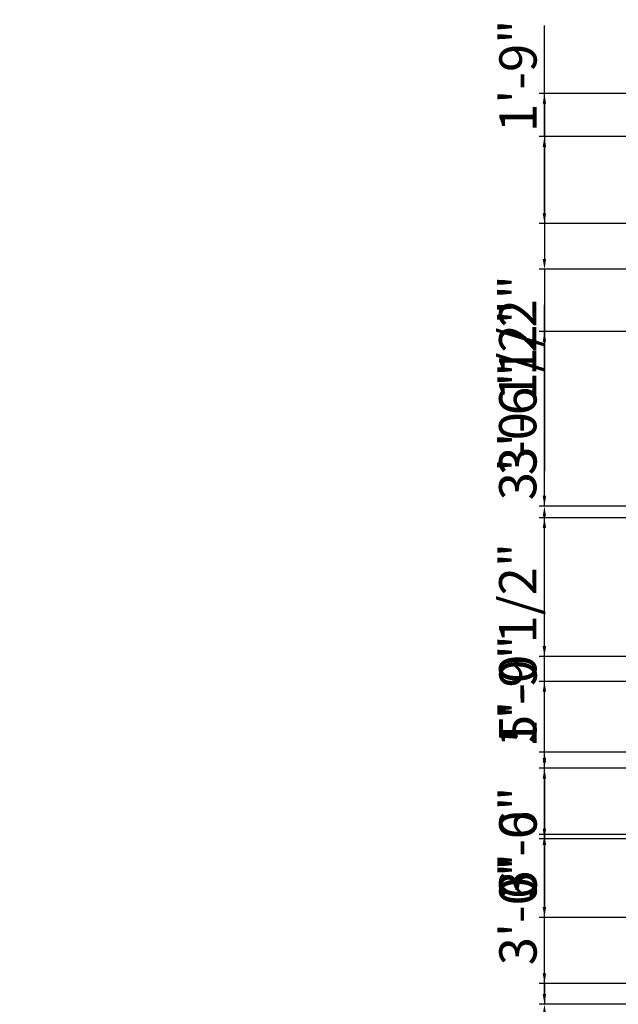
# Model space of a CAD drawing. Units: inches. Extents: x 2181 to 2717, y 1819 to 2296.
# Tile 2 of 5: x 2181 to 2326, y 2036 to 2274. Entities that reach past the tile are written whole.
import ezdxf

# ---------------------------------------------------------------- set-up
doc = ezdxf.new("R2010")
doc.units = ezdxf.units.IN
doc.layers.add('A-ANNO-DIMS', color=2, linetype='Continuous', lineweight=13)
doc.styles.get("Standard").update_dxf_attribs({"font": 'arial.ttf'})
doc.dimstyles.new('ISO-25', dxfattribs={"dimtxt": 9, "dimasz": 2.5, "dimexe": 1.25, "dimexo": 0.625, "dimtad": 1, "dimlunit": 3, "dimtxsty": 'Standard', "dimcen": 2.5, "dimadec": 0, "dimazin": 0, "dimtfac": 1, "dimtmove": 0, "dimatfit": 3, "dimfxl": 1, "dimarcsym": 0})

# ---------------------------------------------------------------- blocks, each defined once
blk = doc.blocks.new('*D19')
at = {"layer": 'A-ANNO-DIMS', "color": 0, "lineweight": -2, "transparency": 16777216}
for p, q in [((2338.35, 1997.93), (2181.23, 1997.93)), ((2338.35, 1986.33), (2338.35, 1999.18)), ((2417.32, 1997.93), (2340.85, 1997.93)), ((2419.82, 1986.33), (2419.82, 1999.18))]:
    blk.add_line(p, q, dxfattribs=at)
at = {"layer": 'A-ANNO-DIMS', "color": 0, "transparency": 16777216}
for points in [[(2340.85, 1998.34), (2340.85, 1997.51), (2338.35, 1997.93)], [(2417.32, 1998.34), (2417.32, 1997.51), (2419.82, 1997.93)]]:
    blk.add_solid(points, dxfattribs=at)
at = {"layer": 'Defpoints', "color": 0, "transparency": 16777216}
for p in [(2338.35, 1997.93), (2338.35, 1985.7), (2419.82, 1985.7)]:
    blk.add_point(p, dxfattribs=at)
at = {"layer": 'A-ANNO-DIMS', "color": 0, "transparency": 16777216, "insert": (2258.54, 2003.48), "char_height": 9, "attachment_point": 5}
blk.add_mtext('QUEEN BED 6\'-9 1/2" TYP.', dxfattribs=at)
blk = doc.blocks.new('*D26')
at = {"layer": 'A-ANNO-DIMS', "color": 0, "lineweight": -2, "transparency": 16777216}
for p, q in [((2328.72, 2256.2), (2306.75, 2256.2)), ((2308, 2253.7), (2308, 2216.2)), ((2328.72, 2213.7), (2306.75, 2213.7)), ((2308, 2213.7), (2308, 2165.07))]:
    blk.add_line(p, q, dxfattribs=at)
at = {"layer": 'A-ANNO-DIMS', "color": 0, "transparency": 16777216}
for points in [[(2307.58, 2253.7), (2308.41, 2253.7), (2308, 2256.2)], [(2307.58, 2216.2), (2308.41, 2216.2), (2308, 2213.7)]]:
    blk.add_solid(points, dxfattribs=at)
at = {"layer": 'Defpoints', "color": 0, "transparency": 16777216}
for p in [(2329.35, 2256.2), (2308, 2213.7), (2329.35, 2213.7)]:
    blk.add_point(p, dxfattribs=at)
at = {"layer": 'A-ANNO-DIMS', "color": 0, "transparency": 16777216, "insert": (2302.71, 2188.13), "char_height": 9, "attachment_point": 5, "rotation": 90}
blk.add_mtext('3\'-6 1/2"', dxfattribs=at)
blk = doc.blocks.new('*D27')
at = {"layer": 'A-ANNO-DIMS', "color": 0, "lineweight": -2, "transparency": 16777216}
for p, q in [((2328.72, 2093.2), (2306.75, 2093.2)), ((2308, 2090.7), (2308, 2059.7)), ((2328.72, 2057.2), (2306.75, 2057.2))]:
    blk.add_line(p, q, dxfattribs=at)
at = {"layer": 'A-ANNO-DIMS', "color": 0, "transparency": 16777216}
for points in [[(2307.58, 2090.7), (2308.41, 2090.7), (2308, 2093.2)], [(2307.58, 2059.7), (2308.41, 2059.7), (2308, 2057.2)]]:
    blk.add_solid(points, dxfattribs=at)
at = {"layer": 'Defpoints', "color": 0, "transparency": 16777216}
for p in [(2329.35, 2093.2), (2308, 2057.2), (2329.35, 2057.2)]:
    blk.add_point(p, dxfattribs=at)
at = {"layer": 'A-ANNO-DIMS', "color": 0, "transparency": 16777216, "insert": (2302.77, 2075.2), "char_height": 9, "attachment_point": 5, "rotation": 90}
blk.add_mtext('3\'-0"', dxfattribs=at)
blk = doc.blocks.new('*D28')
at = {"layer": 'A-ANNO-DIMS', "color": 0, "lineweight": -2, "transparency": 16777216}
for p, q in [((2328.72, 2153.7), (2306.75, 2153.7)), ((2308, 2095.7), (2308, 2151.2)), ((2328.72, 2093.2), (2306.75, 2093.2))]:
    blk.add_line(p, q, dxfattribs=at)
at = {"layer": 'A-ANNO-DIMS', "color": 0, "transparency": 16777216}
for points in [[(2307.58, 2151.2), (2308.41, 2151.2), (2308, 2153.7)], [(2307.58, 2095.7), (2308.41, 2095.7), (2308, 2093.2)]]:
    blk.add_solid(points, dxfattribs=at)
at = {"layer": 'Defpoints', "color": 0, "transparency": 16777216}
for p in [(2308, 2153.7), (2329.35, 2153.7), (2329.35, 2093.2)]:
    blk.add_point(p, dxfattribs=at)
at = {"layer": 'A-ANNO-DIMS', "color": 0, "transparency": 16777216, "insert": (2302.72, 2123.45), "char_height": 9, "attachment_point": 5, "rotation": 90}
blk.add_mtext('5\'-0 1/2"', dxfattribs=at)
blk = doc.blocks.new('*D44')
at = {"layer": 'A-ANNO-DIMS', "color": 0, "lineweight": -2, "transparency": 16777216}
for p, q in [((2308, 2245.76), (2308, 2272.59)), ((2394.49, 2245.76), (2306.75, 2245.76)), ((2308, 2227.26), (2308, 2243.26)), ((2394.49, 2224.76), (2306.75, 2224.76))]:
    blk.add_line(p, q, dxfattribs=at)
at = {"layer": 'A-ANNO-DIMS', "color": 0, "transparency": 16777216}
for points in [[(2307.58, 2243.26), (2308.41, 2243.26), (2308, 2245.76)], [(2307.58, 2227.26), (2308.41, 2227.26), (2308, 2224.76)]]:
    blk.add_solid(points, dxfattribs=at)
at = {"layer": 'Defpoints', "color": 0, "transparency": 16777216}
for p in [(2308, 2245.76), (2395.11, 2245.76), (2395.11, 2224.76)]:
    blk.add_point(p, dxfattribs=at)
at = {"layer": 'A-ANNO-DIMS', "color": 0, "transparency": 16777216, "insert": (2302.78, 2260.43), "char_height": 9, "attachment_point": 5, "rotation": 90}
blk.add_mtext('1\'-9"', dxfattribs=at)
blk = doc.blocks.new('*D46')
at = {"layer": 'A-ANNO-DIMS', "color": 0, "lineweight": -2, "transparency": 16777216}
for p, q in [((2341.24, 2198.7), (2306.75, 2198.7)), ((2308, 2159.01), (2308, 2196.2)), ((2341.24, 2156.51), (2306.75, 2156.51))]:
    blk.add_line(p, q, dxfattribs=at)
at = {"layer": 'A-ANNO-DIMS', "color": 0, "transparency": 16777216}
for points in [[(2307.58, 2196.2), (2308.41, 2196.2), (2308, 2198.7)], [(2307.58, 2159.01), (2308.41, 2159.01), (2308, 2156.51)]]:
    blk.add_solid(points, dxfattribs=at)
at = {"layer": 'Defpoints', "color": 0, "transparency": 16777216}
for p in [(2308, 2198.7), (2341.86, 2198.7), (2341.86, 2156.51)]:
    blk.add_point(p, dxfattribs=at)
at = {"layer": 'A-ANNO-DIMS', "color": 0, "transparency": 16777216, "insert": (2302.77, 2177.61), "char_height": 9, "attachment_point": 5, "rotation": 90}
blk.add_mtext('3\'-6"', dxfattribs=at)
blk = doc.blocks.new('*D48')
at = {"layer": 'A-ANNO-DIMS', "color": 0, "lineweight": -2, "transparency": 16777216}
for p, q in [((2308, 2156.51), (2308, 2205.15)), ((2341.24, 2156.51), (2306.75, 2156.51)), ((2308, 2122.7), (2308, 2154.01)), ((2337.72, 2120.2), (2306.75, 2120.2))]:
    blk.add_line(p, q, dxfattribs=at)
at = {"layer": 'A-ANNO-DIMS', "color": 0, "transparency": 16777216}
for points in [[(2307.58, 2154.01), (2308.41, 2154.01), (2308, 2156.51)], [(2307.58, 2122.7), (2308.41, 2122.7), (2308, 2120.2)]]:
    blk.add_solid(points, dxfattribs=at)
at = {"layer": 'Defpoints', "color": 0, "transparency": 16777216}
for p in [(2308, 2156.51), (2341.86, 2156.51), (2338.35, 2120.2)]:
    blk.add_point(p, dxfattribs=at)
at = {"layer": 'A-ANNO-DIMS', "color": 0, "transparency": 16777216, "insert": (2302.71, 2182.08), "char_height": 9, "attachment_point": 5, "rotation": 90}
blk.add_mtext('3\'-0 1/2"', dxfattribs=at)
blk = doc.blocks.new('*D50')
at = {"layer": 'A-ANNO-DIMS', "color": 0, "lineweight": -2, "transparency": 16777216}
for p, q in [((2308, 2097.13), (2308, 2123.96)), ((2611.72, 2097.13), (2306.75, 2097.13)), ((2308, 2078.63), (2308, 2094.63)), ((2611.72, 2076.13), (2306.75, 2076.13))]:
    blk.add_line(p, q, dxfattribs=at)
at = {"layer": 'A-ANNO-DIMS', "color": 0, "transparency": 16777216}
for points in [[(2307.58, 2094.63), (2308.41, 2094.63), (2308, 2097.13)], [(2307.58, 2078.63), (2308.41, 2078.63), (2308, 2076.13)]]:
    blk.add_solid(points, dxfattribs=at)
at = {"layer": 'Defpoints', "color": 0, "transparency": 16777216}
for p in [(2308, 2097.13), (2612.35, 2097.13), (2612.35, 2076.13)]:
    blk.add_point(p, dxfattribs=at)
at = {"layer": 'A-ANNO-DIMS', "color": 0, "transparency": 16777216, "insert": (2302.78, 2111.79), "char_height": 9, "attachment_point": 5, "rotation": 90}
blk.add_mtext('1\'-9"', dxfattribs=at)
blk = doc.blocks.new('*D52')
at = {"layer": 'A-ANNO-DIMS', "color": 0, "lineweight": -2, "transparency": 16777216}
for p, q in [((2542.72, 2077.19), (2306.75, 2077.19)), ((2308, 2043.69), (2308, 2074.69)), ((2542.72, 2041.19), (2306.75, 2041.19))]:
    blk.add_line(p, q, dxfattribs=at)
at = {"layer": 'A-ANNO-DIMS', "color": 0, "transparency": 16777216}
for points in [[(2307.58, 2074.69), (2308.41, 2074.69), (2308, 2077.19)], [(2307.58, 2043.69), (2308.41, 2043.69), (2308, 2041.19)]]:
    blk.add_solid(points, dxfattribs=at)
at = {"layer": 'Defpoints', "color": 0, "transparency": 16777216}
for p in [(2308, 2077.19), (2543.35, 2077.19), (2543.35, 2041.19)]:
    blk.add_point(p, dxfattribs=at)
at = {"layer": 'A-ANNO-DIMS', "color": 0, "transparency": 16777216, "insert": (2302.77, 2059.19), "char_height": 9, "attachment_point": 5, "rotation": 90}
blk.add_mtext('3\'-0"', dxfattribs=at)
blk = doc.blocks.new('*D53')
at = {"layer": 'A-ANNO-DIMS', "color": 0, "lineweight": -2, "transparency": 16777216}
for p, q in [((2308, 2043.69), (2308, 2046.19)), ((2549.72, 2041.19), (2306.75, 2041.19)), ((2308, 2041.19), (2308, 2036.2)), ((2549.72, 2036.2), (2306.75, 2036.2)), ((2308, 2033.7), (2308, 2006.03))]:
    blk.add_line(p, q, dxfattribs=at)
at = {"layer": 'A-ANNO-DIMS', "color": 0, "transparency": 16777216}
for points in [[(2307.58, 2043.69), (2308.41, 2043.69), (2308, 2041.19)], [(2307.58, 2033.7), (2308.41, 2033.7), (2308, 2036.2)]]:
    blk.add_solid(points, dxfattribs=at)
at = {"layer": 'Defpoints', "color": 0, "transparency": 16777216}
for p in [(2550.35, 2041.19), (2308, 2036.2), (2550.35, 2036.2)]:
    blk.add_point(p, dxfattribs=at)
at = {"layer": 'A-ANNO-DIMS', "color": 0, "transparency": 16777216, "insert": (2302.78, 2018.62), "char_height": 9, "attachment_point": 5, "rotation": 90}
blk.add_mtext('0\'-5"', dxfattribs=at)
blk = doc.blocks.new('*D56')
at = {"layer": 'A-ANNO-DIMS', "color": 0, "lineweight": -2, "transparency": 16777216}
for p, q in [((2549.72, 2114.2), (2306.75, 2114.2)), ((2308, 2038.7), (2308, 2111.7)), ((2549.72, 2036.2), (2306.75, 2036.2))]:
    blk.add_line(p, q, dxfattribs=at)
at = {"layer": 'A-ANNO-DIMS', "color": 0, "transparency": 16777216}
for points in [[(2307.58, 2111.7), (2308.41, 2111.7), (2308, 2114.2)], [(2307.58, 2038.7), (2308.41, 2038.7), (2308, 2036.2)]]:
    blk.add_solid(points, dxfattribs=at)
at = {"layer": 'Defpoints', "color": 0, "transparency": 16777216}
for p in [(2308, 2114.2), (2550.35, 2114.2), (2550.35, 2036.2)]:
    blk.add_point(p, dxfattribs=at)
at = {"layer": 'A-ANNO-DIMS', "color": 0, "transparency": 16777216, "insert": (2302.78, 2075.2), "char_height": 9, "attachment_point": 5, "rotation": 90}
blk.add_mtext('6\'-6"', dxfattribs=at)

msp = doc.modelspace()

# ---------------------------------------------------------------- dimensions: what is measured, and where the dimension line sits
at = {"layer": 'A-ANNO-DIMS'}
for base, p1, p2, picture, middle in [((2307.996, 2245.763), (2395.11, 2224.763), (2395.11, 2245.763), '*D44', (2302.776, 2260.426)), ((2307.996, 2213.705), (2329.346, 2256.205), (2329.346, 2213.705), '*D26', (2302.715, 2188.135)), ((2307.996, 2156.51), (2338.346, 2120.205), (2341.861, 2156.51), '*D48', (2302.715, 2182.08)), ((2307.996, 2198.704), (2341.861, 2156.51), (2341.861, 2198.704), '*D46', (2302.773, 2177.607)), ((2307.996, 2153.705), (2329.346, 2093.205), (2329.346, 2153.705), '*D28', (2302.718, 2123.455)), ((2307.996, 2097.128), (2612.346, 2076.128), (2612.346, 2097.128), '*D50', (2302.776, 2111.792)), ((2307.996, 2114.205), (2550.346, 2036.205), (2550.346, 2114.205), '*D56', (2302.776, 2075.205)), ((2307.996, 2057.205), (2329.346, 2093.205), (2329.346, 2057.205), '*D27', (2302.773, 2075.205)), ((2307.996, 2077.187), (2543.346, 2041.187), (2543.346, 2077.187), '*D52', (2302.773, 2059.187)), ((2307.996, 2036.205), (2550.346, 2041.187), (2550.346, 2036.205), '*D53', (2302.776, 2018.617))]:
    dim = msp.add_linear_dim(base=base, p1=p1, p2=p2, angle=90, dimstyle='ISO-25', override={"dimdec": 1, "dimlfac": 1, "dimrnd": 0, "dimzin": 1, "dimdsep": 46, "dimlunit": 4, "dimfrac": 2}, dxfattribs=at)
    dim.commit()
    dim.dimension.update_dxf_attribs({"geometry": picture, "text_midpoint": middle})
dim = msp.add_linear_dim(base=(2338.346, 1997.926), p1=(2419.819, 1985.705), p2=(2338.346, 1985.705), angle=180, text='QUEEN BED <> TYP.', dimstyle='ISO-25', override={"dimdec": 1, "dimlfac": 1, "dimrnd": 0, "dimzin": 1, "dimdsep": 46, "dimlunit": 4, "dimfrac": 2}, dxfattribs=at)
dim.commit()
dim.dimension.update_dxf_attribs({"geometry": '*D19', "text_midpoint": (2258.54, 2003.48)})

doc.saveas('drawing.dxf')
